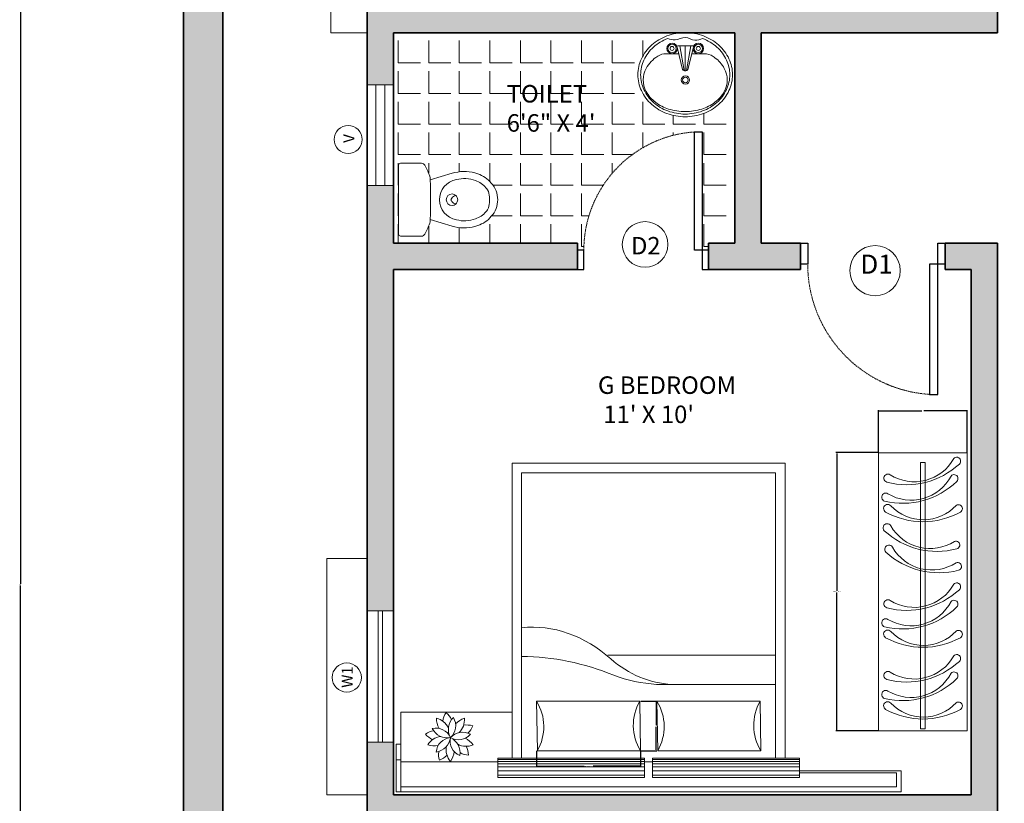
# Model space of a CAD drawing. Units: inches. Extents: x 2701 to 6846, y 811 to 2447.
# Tile 7 of 20: x 2701 to 2926, y 1130 to 1309. Entities that reach past the tile are written whole.
import ezdxf

# ---------------------------------------------------------------- set-up
doc = ezdxf.new("R2010")
doc.units = ezdxf.units.IN
doc.linetypes.add('HIDDEN4', pattern=[0.09375, 0.0625, -0.03125])
for name, color, linetype, lineweight in [('A-ANNO-DIMS', 2, 'Continuous', 18), ('A-ANNO-IDEN', 7, 'Continuous', 13), ('A-AREA-IDEN', 7, 'Continuous', 18), ('A-DOOR', 4, 'Continuous', 25), ('A-DOOR-SWNG', 4, 'HIDDEN4', 13), ('A-FLOR-FIXT', 7, 'Continuous', 18), ('A-FLOR-PATT', 252, 'Continuous', 13), ('A-FURN', 8, 'Continuous', 13), ('A-GLAZ', 4, 'Continuous', 18), ('A-WALL', 7, 'Continuous', 35), ('C-PROP', 7, 'Continuous', 35)]:
    doc.layers.add(name, color=color, linetype=linetype, lineweight=lineweight)
doc.layers.add('A-WALL-PATT', color=18, linetype='Continuous', lineweight=13, true_color=0x000000)
doc.layers.add('C-PROP-PATT', color=18, linetype='Continuous', lineweight=13, true_color=0x000000)
doc.styles.get("Standard").update_dxf_attribs({"font": 'arial.ttf'})
doc.dimstyles.get("Standard").update_dxf_attribs({"dimtxt": 0.18, "dimasz": 0.18, "dimexe": 0.18, "dimexo": 0.0625, "dimgap": 0.09, "dimtad": 0, "dimtih": 1, "dimtoh": 1, "dimdec": 4, "dimzin": 0, "dimdsep": 46, "dimtxsty": 'Standard', "dimcen": 0.09, "dimadec": 0, "dimazin": 0, "dimtfac": 1, "dimtdec": 4, "dimtofl": 0, "dimtmove": 0, "dimatfit": 3, "dimfxl": 1, "dimtolj": 1, "dimtzin": 0, "dimarcsym": 0})

# ---------------------------------------------------------------- blocks, each defined once
blk = doc.blocks.new('V')
for p, q in [((3304.15, 1279.33), (3281.15, 1279.33)), ((3304.15, 1277.33), (3281.15, 1277.33)), ((3304.15, 1275.33), (3281.15, 1275.33)), ((3281.15, 1273.33), (3304.15, 1273.33))]:
    blk.add_line(p, q)
blk.add_circle((3293.67, 1283.69), 3.19)
at = {"insert": (3292.45, 1284.76), "char_height": 2.5, "attachment_point": 1}
blk.add_mtext_dynamic_manual_height_columns('V', width=0.0153, gutter_width=12.5, heights=[0], dxfattribs=at)
blk = doc.blocks.new('V1')
for p, q in [((3281.15, 1279.33), (3281.15, 1273.33)), ((3304.15, 1273.33), (3304.15, 1279.33))]:
    blk.add_line(p, q)
blk.add_blockref('V', (0, 0))
blk = doc.blocks.new('A$C20D7642B')
for p, q in [((0, 1879.7), (0, 0)), ((600, 1879.7), (0, 1879.7)), ((600, 1879.7), (600, 0)), ((285.2, 14), (285.2, 1812.3)), ((285.2, 1812.3), (316, 1812.3)), ((316, 1812.3), (316, 14)), ((340, 0), (0, 0)), ((316, 14), (285.2, 14)), ((340, 0), (600, 0))]:
    blk.add_line(p, q)
for centre, radius, start, end in [((189.7, 2189.4), 526.2, 255.30638, 312.74923), ((242.6, 1988.3), 305.1, 237.78554, 330.91711), ((529.2, 1822.6), 26.4, 312.06888, 138.87685), ((64.5, 1707), 27.8, 56.33784, 252.73759), ((511.2, 1705.1), 26.4, 313.4541, 140.26207), ((163, 2063.5), 526.2, 256.69161, 314.13445), ((220.7, 1863.8), 305.1, 239.17077, 332.30233), ((49.5, 1578.3), 27.8, 57.72306, 254.12281), ((62.8, 1501.9), 27.8, 42.31003, 238.70978), ((301.2, 1939.5), 526.2, 241.27858, 298.72142), ((303.8, 1731.6), 305.1, 223.75774, 316.8893), ((541.6, 1501.4), 26.4, 298.04107, 124.84904), ((59.1, 1372.1), 27.8, 28.28014, 224.67989), ((396.5, 1738.9), 526.2, 227.24868, 284.69153), ((348.6, 1536.6), 305.1, 209.72784, 302.85941), ((523.6, 1255.6), 26.4, 284.01118, 110.81915), ((70.6, 1227.4), 27.8, 28.28014, 224.67989), ((408, 1594.2), 526.2, 227.24868, 284.69153), ((360, 1391.9), 305.1, 209.72784, 302.85941), ((535, 1110.9), 26.4, 284.01118, 110.81915), ((529.2, 973.6), 26.4, 312.06888, 138.87685), ((189.7, 1340.3), 526.2, 255.30638, 312.74923), ((242.6, 1139.3), 305.1, 237.78554, 330.91711), ((64.5, 857.9), 27.8, 56.33784, 252.73759), ((220.7, 1014.8), 305.1, 239.17077, 332.30233), ((511.2, 856), 26.4, 313.4541, 140.26207), ((163, 1214.5), 526.2, 256.69161, 314.13445), ((49.5, 729.2), 27.8, 57.72306, 254.12281), ((62.8, 652.8), 27.8, 42.31003, 238.70978), ((303.8, 882.6), 305.1, 223.75774, 316.8893), ((541.6, 652.4), 26.4, 298.04107, 124.84904), ((301.2, 1090.5), 526.2, 241.27858, 298.72142), ((189.7, 856), 526.2, 255.30638, 312.74923), ((242.6, 655), 305.1, 237.78554, 330.91711), ((529.2, 489.2), 26.4, 312.06888, 138.87685), ((64.5, 373.6), 27.8, 56.33784, 252.73759), ((163, 730.2), 526.2, 256.69161, 314.13445), ((220.7, 530.5), 305.1, 239.17077, 332.30233), ((511.2, 371.7), 26.4, 313.4541, 140.26207), ((49.5, 244.9), 27.8, 57.72306, 254.12281), ((62.8, 168.5), 27.8, 42.31003, 238.70978), ((301.2, 606.1), 526.2, 241.27858, 298.72142), ((303.8, 398.3), 305.1, 223.75774, 316.8893), ((541.6, 168), 26.4, 298.04107, 124.84904)]:
    blk.add_arc(centre, radius, start, end)
blk = doc.blocks.new('A$C62EA08CE')
at = {"linetype": 'ByBlock'}
for p, q in [((0.2191, 0.3943), (0.3067, 0.3943)), ((0.2328, 0.3943), (0.2566, 0.2566)), ((0.2629, 0.3943), (0.2629, 0.2555)), ((0.2933, 0.3943), (0.2696, 0.2568)), ((0.1569, 0.3505), (0.2264, 0.3505)), ((0.2191, 0.3797), (0.2483, 0.2629)), ((0.2775, 0.2629), (0.3067, 0.3797)), ((0.2994, 0.3505), (0.3691, 0.3505))]:
    blk.add_line(p, q, dxfattribs=at)
for centre, radius in [((0.1899, 0.3797), 0.0292), ((0.1899, 0.3797), 0.0232), ((0.1899, 0.3797), 0.0112), ((0.3359, 0.3797), 0.0292), ((0.3359, 0.3797), 0.0232), ((0.3359, 0.3797), 0.0112), ((0.264, 0.2045), 0.0234), ((0.264, 0.2045), 0.0154)]:
    blk.add_circle(centre, radius, dxfattribs=at)
for centre, radius, start, end in [((0.2518, 0.2022), 0.2632, 110.2132, 131.6335), ((0.2629, 0.1722), 0.2952, 90, 110.2132), ((0.2629, 0.1722), 0.2952, 69.7868, 90), ((0.2739, 0.2022), 0.2632, 48.3665, 69.7868), ((0.2348, 0.2214), 0.2375, 131.6335, 155.0149), ((0.2348, 0.2214), 0.2225, 131.6335, 155.0149), ((0.2518, 0.2022), 0.2482, 110.2132, 131.6335), ((0.2739, 0.2022), 0.2482, 48.3665, 69.7868), ((0.291, 0.2214), 0.2225, 24.9851, 48.3665), ((0.291, 0.2214), 0.2375, 24.9851, 48.3665), ((0.2107, 0.1777), 0.1883, 122.2598, 151.0888), ((0.1569, 0.2629), 0.0876, 90, 122.2598), ((0.3691, 0.2629), 0.0876, 56.0955, 90), ((0.2835, 0.1356), 0.241, 53.1301, 56.0955), ((0.2084, 0.2337), 0.2084, 155.0149, 180), ((0.2084, 0.2337), 0.1934, 155.0149, 180), ((0.3151, 0.1777), 0.1883, 28.9112, 53.1301), ((0.3174, 0.2337), 0.1934, 360, 24.9851), ((0.3174, 0.2337), 0.2084, 360, 24.9851), ((0.2084, 0.2337), 0.2084, 180, 204.9851), ((0.2084, 0.2337), 0.1934, 180, 204.9851), ((0.1622, 0.2045), 0.133, 151.0888, 180), ((0.2629, 0.2737), 0.0182, 216.4225, 323.5775), ((0.3636, 0.2045), 0.133, 0, 28.9112), ((0.3174, 0.2337), 0.1934, 335.0149, 0), ((0.3174, 0.2337), 0.2084, 335.0149, 0), ((0.1622, 0.2045), 0.133, 180, 208.9112), ((0.3636, 0.2045), 0.133, 331.0888, 0), ((0.2348, 0.246), 0.2375, 204.9851, 228.3665), ((0.2348, 0.246), 0.2225, 204.9851, 228.3665), ((0.2107, 0.2312), 0.1883, 208.9112, 233.1301), ((0.3151, 0.2312), 0.1883, 306.8699, 331.0888), ((0.291, 0.246), 0.2225, 311.6335, 335.0149), ((0.291, 0.246), 0.2375, 311.6335, 335.0149), ((0.2518, 0.2651), 0.2632, 228.3665, 249.7868), ((0.2518, 0.2651), 0.2482, 228.3665, 249.7868), ((0.2423, 0.2733), 0.241, 233.1301, 252.7421), ((0.2835, 0.2733), 0.241, 287.2579, 306.8699), ((0.2739, 0.2651), 0.2482, 290.2132, 311.6335), ((0.2739, 0.2651), 0.2632, 290.2132, 311.6335), ((0.2629, 0.2952), 0.2952, 249.7868, 270), ((0.2629, 0.2952), 0.2802, 249.7868, 270), ((0.2629, 0.3398), 0.3106, 252.7421, 270), ((0.2629, 0.3398), 0.3106, 270, 287.2579), ((0.2629, 0.2952), 0.2802, 270, 290.2132), ((0.2629, 0.2952), 0.2952, 270, 290.2132)]:
    blk.add_arc(centre, radius, start, end, dxfattribs=at)
blk.add_open_spline([(0.1661, 0.4351), (0.1795, 0.4306), (0.2124, 0.4195), (0.2631, 0.4543), (0.3132, 0.4162), (0.3455, 0.4293), (0.3597, 0.4351)], degree=3, knots=[0, 0, 0, 0, 0.0411087, 0.1003374, 0.1559132, 0.1995858, 0.1995858, 0.1995858, 0.1995858], dxfattribs=at)
blk = doc.blocks.new('A$C150B42AD')
at = {"ltscale": 20}
for p, q in [((0.243, 0.6605), (0.0125, 0.6605)), ((0.243, 0.6605), (0.4735, 0.6605)), ((0, 0.648), (0, 0.508)), ((0.486, 0.648), (0.486, 0.508)), ((0.11, 0.4499), (0.067, 0.3038)), ((0.1071, 0.45), (0.1511, 0.4485)), ((0.1511, 0.4485), (0.243, 0.4485)), ((0.3349, 0.4485), (0.243, 0.4485)), ((0.3789, 0.45), (0.3349, 0.4485)), ((0.376, 0.4499), (0.419, 0.3038)), ((0.2245, 0.0549), (0.243, 0.0549)), ((0.2615, 0.0549), (0.243, 0.0549))]:
    blk.add_line(p, q, dxfattribs=at)
for centre, radius, start, end in [((0.0125, 0.648), 0.0125, 90, 180), ((0.4735, 0.648), 0.0125, 0, 90), ((0.024, 0.508), 0.024, 180, 244), ((0.2288, 0.8612), 0.4323, 240.11805, 247.88195), ((0.1119, 0.5519), 0.102, 243.30484, 267.30484), ((0.3741, 0.5519), 0.102, 272.69516, 296.69516), ((0.2572, 0.8612), 0.4323, 292.11805, 299.88195), ((0.462, 0.508), 0.024, 296, 0), ((0.243, 0.252), 0.136, 90, 170.10936), ((0.243, 0.3047), 0.0384, 90, 270), ((0.243, 0.252), 0.136, 9.89064, 90), ((0.243, 0.3047), 0.0384, 270, 90), ((0.3111, 0.2222), 0.2565, 165.7118, 200.33768), ((0.243, 0.252), 0.1835, 163.59952, 169.46851), ((0.3111, 0.2222), 0.209, 165.27447, 200.60776), ((0.2251, 0.2822), 0.00957, 149.18444, 231.80771), ((0.2645, 0.2649), 0.0525, 119.17381, 155.01561), ((0.2439, 0.2978), 0.0139, 93.65397, 111.19045), ((0.2421, 0.2978), 0.0139, 68.80955, 86.34603), ((0.2215, 0.2649), 0.0525, 24.98439, 60.82619), ((0.2609, 0.2822), 0.00957, 308.19229, 30.81556), ((0.1749, 0.2222), 0.209, 339.39224, 14.72553), ((0.1749, 0.2222), 0.2565, 339.66232, 14.2882), ((0.243, 0.252), 0.1835, 10.53149, 16.40048), ((0.258, 0.194), 0.197, 198.0034, 230.27404), ((0.258, 0.194), 0.1495, 197.63909, 230.62819), ((0.228, 0.194), 0.1495, 309.37181, 342.36091), ((0.228, 0.194), 0.197, 309.72596, 341.9966), ((0.243, 0.166), 0.1185, 227.64547, 235.84675), ((0.2245, 0.1499), 0.095, 239.63238, 270), ((0.2615, 0.1499), 0.095, 270, 300.36762), ((0.243, 0.166), 0.1185, 304.15325, 312.35453), ((0.243, 0.166), 0.166, 228.0788, 270), ((0.243, 0.166), 0.166, 270, 311.9212)]:
    blk.add_arc(centre, radius, start, end, dxfattribs=at)
blk = doc.blocks.new('DOOR-D1-33IN-PANEL-FRAME')
blk.add_lwpolyline([(0, 33), (0, 31.37), (4.8, 31.37), (4.8, 33), (0, 33)], close=True)
for points in [[(4.32, 33), (0.48, 33)], [(4.8, 0), (4.8, 3.55), (34.54, 3.55), (34.54, 1.63), (0, 1.63), (0, 0)], [(0, 0), (4.8, 0)], [(4.32, 0), (0.48, 0)]]:
    blk.add_lwpolyline(points)
blk = doc.blocks.new('DOOR-D2-30IN-PANEL-FRAME')
blk.add_lwpolyline([(0, 30), (0, 28.52), (4.36, 28.52), (4.36, 30), (0, 30)], close=True)
for points in [[(3.93, 30), (0.44, 30)], [(4.36, 0), (4.36, 3.22), (31.4, 3.22), (31.4, 1.48), (0, 1.48), (0, 0)], [(0, 0), (4.36, 0)], [(3.93, 0), (0.44, 0)]]:
    blk.add_lwpolyline(points)
blk = doc.blocks.new('BED-PILLOW')
for p, q in [((23.58, 11.3), (0, 11.3)), ((0, 11.3), (0.17, 0)), ((23.75, 0), (23.58, 11.3)), ((0.17, 0), (23.75, 0))]:
    blk.add_line(p, q)
for centre, start, end in [((-9.32, 5.51), 329.8722, 31.8713), ((33.07, 5.79), 149.8722, 211.8713)]:
    blk.add_arc(centre, 10.97, start, end)
blk = doc.blocks.new('*D43')
at = {"layer": 'A-ANNO-DIMS', "color": 0, "lineweight": -2, "transparency": 16777216}
for p, q in [((2896.7, 1210.2), (2887.05, 1210.2)), ((2887.23, 1210.02), (2887.23, 1178.62)), ((2887.23, 1146.85), (2887.23, 1178.25)), ((2896.7, 1146.67), (2887.05, 1146.67))]:
    blk.add_line(p, q, dxfattribs=at)
at = {"layer": 'A-ANNO-DIMS', "color": 0, "transparency": 16777216}
for points in [[(2887.2, 1210.02), (2887.26, 1210.02), (2887.23, 1210.2)], [(2887.2, 1146.85), (2887.26, 1146.85), (2887.23, 1146.67)]]:
    blk.add_solid(points, dxfattribs=at)
at = {"layer": 'Defpoints', "color": 0, "transparency": 16777216}
for p in [(2887.23, 1210.2), (2896.76, 1210.2), (2896.76, 1146.67)]:
    blk.add_point(p, dxfattribs=at)
at = {"layer": 'A-ANNO-DIMS', "color": 0, "transparency": 16777216, "insert": (2887.23, 1178.44), "char_height": 0.18, "attachment_point": 5}
blk.add_mtext('\\A1;WARDROBE 64', dxfattribs=at)
blk = doc.blocks.new('*D44')
at = {"layer": 'A-ANNO-DIMS', "color": 0, "lineweight": -2, "transparency": 16777216}
for p, q in [((2896.76, 1210.26), (2896.76, 1219.91)), ((2896.94, 1219.73), (2906.68, 1219.73)), ((2916.86, 1219.73), (2907.12, 1219.73)), ((2917.04, 1210.26), (2917.04, 1219.91))]:
    blk.add_line(p, q, dxfattribs=at)
at = {"layer": 'A-ANNO-DIMS', "color": 0, "transparency": 16777216}
for points in [[(2896.94, 1219.76), (2896.94, 1219.7), (2896.76, 1219.73)], [(2916.86, 1219.76), (2916.86, 1219.7), (2917.04, 1219.73)]]:
    blk.add_solid(points, dxfattribs=at)
at = {"layer": 'Defpoints', "color": 0, "transparency": 16777216}
for p in [(2917.04, 1219.73), (2896.76, 1210.2), (2917.04, 1210.2)]:
    blk.add_point(p, dxfattribs=at)
at = {"layer": 'A-ANNO-DIMS', "color": 0, "transparency": 16777216, "insert": (2906.9, 1219.73), "char_height": 0.18, "attachment_point": 5}
blk.add_mtext('\\A1;20', dxfattribs=at)
blk = doc.blocks.new('*D47')
at = {"layer": 'A-ANNO-DIMS', "color": 0, "lineweight": -2, "transparency": 16777216}
for p, q in [((2818.66, 1142.07), (2818.66, 1138.39)), ((2842.41, 1142.07), (2842.41, 1138.39)), ((2818.84, 1138.57), (2829.5, 1138.57)), ((2842.23, 1138.57), (2831.57, 1138.57))]:
    blk.add_line(p, q, dxfattribs=at)
at = {"layer": 'A-ANNO-DIMS', "color": 0, "transparency": 16777216}
for points in [[(2818.84, 1138.6), (2818.84, 1138.54), (2818.66, 1138.57)], [(2842.23, 1138.6), (2842.23, 1138.54), (2842.41, 1138.57)]]:
    blk.add_solid(points, dxfattribs=at)
at = {"layer": 'Defpoints', "color": 0, "transparency": 16777216}
for p in [(2818.66, 1142.13), (2842.41, 1142.13), (2842.41, 1138.57)]:
    blk.add_point(p, dxfattribs=at)
at = {"layer": 'A-ANNO-DIMS', "color": 0, "transparency": 16777216, "insert": (2830.53, 1138.57), "char_height": 0.18, "attachment_point": 5}
blk.add_mtext('\\A1;PILLOW 24 TYP.', dxfattribs=at)
blk = doc.blocks.new('*D48')
at = {"layer": 'A-ANNO-DIMS', "color": 0, "lineweight": -2, "transparency": 16777216}
for p, q in [((2842.47, 1153.44), (2846.15, 1153.44)), ((2845.97, 1153.26), (2845.97, 1147.97)), ((2845.97, 1142.31), (2845.97, 1147.61)), ((2842.47, 1142.13), (2846.15, 1142.13))]:
    blk.add_line(p, q, dxfattribs=at)
at = {"layer": 'A-ANNO-DIMS', "color": 0, "transparency": 16777216}
for points in [[(2845.94, 1153.26), (2846, 1153.26), (2845.97, 1153.44)], [(2845.94, 1142.31), (2846, 1142.31), (2845.97, 1142.13)]]:
    blk.add_solid(points, dxfattribs=at)
at = {"layer": 'Defpoints', "color": 0, "transparency": 16777216}
for p in [(2842.41, 1153.44), (2845.97, 1153.44), (2842.41, 1142.13)]:
    blk.add_point(p, dxfattribs=at)
at = {"layer": 'A-ANNO-DIMS', "color": 0, "transparency": 16777216, "insert": (2845.97, 1147.79), "char_height": 0.18, "attachment_point": 5}
blk.add_mtext('\\A1;11 TYP.', dxfattribs=at)
blk = doc.blocks.new('*D66')
at = {"layer": 'A-ANNO-DIMS', "color": 0, "lineweight": -2, "transparency": 16777216}
for p, q in [((2737.91, 1504.05), (2700.59, 1504.05)), ((2700.77, 1503.87), (2700.77, 1180.23)), ((2700.77, 856.23), (2700.77, 1179.87)), ((2737.91, 856.05), (2700.59, 856.05))]:
    blk.add_line(p, q, dxfattribs=at)
at = {"layer": 'A-ANNO-DIMS', "color": 0, "transparency": 16777216}
for points in [[(2700.74, 1503.87), (2700.8, 1503.87), (2700.77, 1504.05)], [(2700.74, 856.23), (2700.8, 856.23), (2700.77, 856.05)]]:
    blk.add_solid(points, dxfattribs=at)
at = {"layer": 'Defpoints', "color": 0, "transparency": 16777216}
for p in [(2700.77, 1504.05), (2737.97, 1504.05), (2737.97, 856.05)]:
    blk.add_point(p, dxfattribs=at)
at = {"layer": 'A-ANNO-DIMS', "color": 0, "transparency": 16777216, "insert": (2700.77, 1180.05), "char_height": 0.18, "attachment_point": 5}
blk.add_mtext('\\A1;648', dxfattribs=at)

msp = doc.modelspace()

# ---------------------------------------------------------------- hatches: boundary and pattern name
at = {"layer": 'A-FLOR-PATT'}
h = msp.add_hatch(dxfattribs=at)
h.set_pattern_fill('ANGLE', color=256)
h.set_pattern_definition([(0, (0, 0), (0, 6.985), [5.08, -1.905]), (90, (0, 0), (-6.985, 4e-16), [5.08, -1.905])])
h.paths.add_polyline_path([(2841.81, 1296.51, -0.109453), (2842.61, 1300.13, -0.102375), (2844.98, 1303.3, -0.093743), (2848.43, 1305.37, -0.062463), (2851.37, 1306.05), (2785.97, 1306.05), (2785.97, 1258.05), (2827.97, 1258.05), (2827.97, 1256.41), (2829.45, 1256.41, -0.394827), (2854.75, 1283.45), (2856.49, 1283.45), (2856.49, 1256.41), (2857.97, 1256.41), (2857.97, 1258.05), (2863.97, 1258.05), (2863.97, 1306.05), (2853.87, 1306.05, -0.062463), (2856.81, 1305.37, -0.093743), (2860.26, 1303.3, -0.102375), (2862.62, 1300.13, -0.109453), (2863.42, 1296.51, -0.109453), (2862.62, 1292.89, -0.102375), (2860.26, 1289.72, -0.093738), (2856.81, 1287.65, -0.088425), (2852.62, 1286.91, -0.088425), (2848.43, 1287.65, -0.093738), (2844.98, 1289.72, -0.102375), (2842.61, 1292.89, -0.109453)])
h.paths.add_polyline_path([(2805.21, 1273.88, -0.141745), (2808.32, 1271.77, -0.184983), (2809.77, 1267.97, -0.184983), (2808.32, 1264.18, -0.141745), (2805.21, 1262.07, -0.152244), (2799.99, 1261.8, -0.025614), (2799.37, 1261.95), (2794.37, 1263.42), (2794.36, 1263.41, -0.111242), (2793.99, 1261.92, -0.033889), (2793.11, 1260.11, -0.286745), (2792.38, 1259.65), (2787.58, 1259.65, -0.414214), (2787.15, 1260.08), (2787.15, 1267.97), (2787.15, 1275.87, -0.414214), (2787.58, 1276.3), (2792.38, 1276.3, -0.286745), (2793.11, 1275.83, -0.033889), (2793.99, 1274.03, -0.105104), (2794.36, 1272.63), (2794.37, 1272.53), (2799.37, 1274, -0.025614), (2799.99, 1274.15, -0.152244)], flags=16)
h.paths.add_polyline_path([(2804.68, 1272.34, -0.144945), (2807.09, 1270.71, -0.0358), (2807.45, 1270.25, -0.133285), (2807.89, 1268.61), (2807.89, 1267.97), (2807.89, 1267.34, -0.133285), (2807.45, 1265.7, -0.0358), (2807.09, 1265.24, -0.144945), (2804.68, 1263.61, -0.155404), (2800.34, 1263.39, -0.364511), (2796.49, 1267.97, -0.364511), (2800.34, 1272.56, -0.155404)], flags=0)
h.paths.add_polyline_path([(2800.02, 1268.9, 0.169298), (2799.13, 1268.12, 0.076667), (2799.1, 1267.97, 0.076667), (2799.13, 1267.83, 0.169298), (2800.02, 1267.05, 0.305219), (2800.37, 1267.16, 0.169535), (2800.65, 1267.97, 0.169535), (2800.37, 1268.79, 0.305219)], flags=0)
h.paths.add_polyline_path([(2971.97, 1456.05), (2923.97, 1456.05), (2923.97, 1408.05), (2922.33, 1408.05), (2922.33, 1406.57, -0.394827), (2949.37, 1381.27), (2949.37, 1379.53), (2922.33, 1379.53), (2922.33, 1378.05), (2923.97, 1378.05), (2923.97, 1372.05), (2971.97, 1372.05)])
h.paths.add_polyline_path([(2939.82, 1436.53, -0.141745), (2937.71, 1433.42, -0.184983), (2933.91, 1431.97, -0.184983), (2930.12, 1433.42, -0.141745), (2928.01, 1436.53, -0.152244), (2927.74, 1441.75, -0.025614), (2927.89, 1442.37), (2929.36, 1447.38), (2929.35, 1447.38, -0.111242), (2927.86, 1447.75, -0.033889), (2926.05, 1448.63, -0.286745), (2925.59, 1449.37), (2925.59, 1454.16, -0.414214), (2926.02, 1454.59), (2933.91, 1454.59), (2941.81, 1454.59, -0.414207), (2942.24, 1454.16), (2942.24, 1449.37, -0.286745), (2941.78, 1448.63, -0.033889), (2939.97, 1447.75, -0.105104), (2938.57, 1447.38), (2938.47, 1447.38), (2939.94, 1442.37, -0.025614), (2940.09, 1441.75, -0.152244)], flags=16)
h.paths.add_polyline_path([(2938.28, 1437.06, -0.144945), (2936.65, 1434.65, -0.0358), (2936.19, 1434.29, -0.133285), (2934.55, 1433.85), (2933.91, 1433.85), (2933.28, 1433.85, -0.133285), (2931.64, 1434.29, -0.0358), (2931.18, 1434.65, -0.144945), (2929.55, 1437.06, -0.155404), (2929.33, 1441.4, -0.364511), (2933.91, 1445.26, -0.364511), (2938.5, 1441.4, -0.155404)], flags=0)
h.paths.add_polyline_path([(2969.16, 1392.04, -0.093743), (2971.22, 1388.6, -0.088421), (2971.97, 1384.4, -0.088421), (2971.22, 1380.21, -0.093743), (2969.16, 1376.76, -0.102375), (2965.99, 1374.4, -0.109453), (2962.37, 1373.6, -0.109453), (2958.75, 1374.4, -0.102375), (2955.58, 1376.76, -0.093738), (2953.51, 1380.21, -0.088425), (2952.76, 1384.4, -0.088425), (2953.51, 1388.6, -0.093738), (2955.58, 1392.04, -0.102375), (2958.75, 1394.41, -0.109453), (2962.37, 1395.21, -0.109453), (2965.99, 1394.41, -0.102375)], flags=0)
edge = h.paths.add_edge_path(flags=16)
edge.add_arc((2961.07, 1384.86), 10.2, 20.2132, 41.6336, ccw=False)
edge.add_spline(control_points=[(2970.65, 1388.38), (2970.46, 1387.83), (2970, 1386.48), (2971.44, 1384.4), (2969.87, 1382.34), (2970.41, 1381.01), (2970.65, 1380.43)], knot_values=[0, 0, 0, 0, 0.041109, 0.100337, 0.155913, 0.199586, 0.199586, 0.199586, 0.199586], degree=3, periodic=0)
edge.add_arc((2961.07, 1383.95), 10.2, 318.3664, 339.7868, ccw=False)
edge.add_arc((2961.86, 1383.25), 9.15, 294.9853, 318.3664, ccw=False)
edge.add_arc((2962.37, 1382.17), 7.95, 270, 294.9853, ccw=False)
edge.add_arc((2962.37, 1382.17), 7.95, 245.0147, 270, ccw=False)
edge.add_arc((2962.87, 1383.25), 9.15, 221.6336, 245.0147, ccw=False)
edge.add_arc((2963.66, 1383.95), 10.2, 200.213, 221.6336, ccw=False)
edge.add_arc((2964.89, 1384.4), 11.51, 180, 200.213, ccw=False)
edge.add_arc((2964.89, 1384.4), 11.51, 159.787, 180, ccw=False)
edge.add_arc((2963.66, 1384.86), 10.2, 138.3664, 159.787, ccw=False)
edge.add_arc((2962.87, 1385.56), 9.15, 114.9853, 138.3664, ccw=False)
edge.add_arc((2962.37, 1386.64), 7.95, 90, 114.9853, ccw=False)
edge.add_arc((2962.37, 1386.64), 7.95, 65.0147, 90, ccw=False)
edge.add_arc((2961.86, 1385.56), 9.15, 41.6336, 65.0147, ccw=False)
h.paths.add_polyline_path([(2963.81, 1393.33, -0.126458), (2966.61, 1390.68, -0.141697), (2967.17, 1388.76), (2967.17, 1387.41, -1), (2969.57, 1387.41, -0.414214), (2968.37, 1386.21), (2963.57, 1385, 0.146218), (2963.31, 1384.66), (2968.97, 1385.64), (2968.97, 1383.15), (2963.32, 1384.13, 0.140312), (2963.57, 1383.8), (2968.37, 1382.6, -0.414214), (2969.57, 1381.4, -1), (2967.17, 1381.4), (2967.17, 1380.04, -0.149025), (2966.56, 1378.03, -0.012759), (2966.26, 1377.62, -0.106303), (2963.81, 1375.48, -0.126822), (2961.17, 1374.8, -0.126822), (2958.52, 1375.48, -0.106303), (2956.07, 1377.62, -0.085722), (2954.54, 1380.62, -0.075351), (2953.96, 1384.4, -0.075351), (2954.54, 1388.19, -0.085722), (2956.07, 1391.19, -0.106303), (2958.52, 1393.33, -0.126822), (2961.17, 1394.01, -0.126822)], flags=0)
h.paths.add_polyline_path([(2934.84, 1441.73, 0.169298), (2934.06, 1442.61, 0.076667), (2933.91, 1442.64, 0.076667), (2933.77, 1442.61, 0.169298), (2932.99, 1441.73, 0.305219), (2933.1, 1441.38, 0.169535), (2933.91, 1441.09, 0.169535), (2934.73, 1441.38, 0.305219)], flags=0)
h.paths.add_polyline_path([(2969.32, 1387.41, -1), (2967.42, 1387.41, -1)], flags=0)
h.paths.add_polyline_path([(2968.83, 1387.41, -1), (2967.91, 1387.41, -1)], flags=0)
h.paths.add_polyline_path([(2962.13, 1384.36, -1), (2960.21, 1384.36, -1)], flags=0)
h.paths.add_polyline_path([(2961.8, 1384.36, -1), (2960.54, 1384.36, -1)], flags=0)
h.paths.add_polyline_path([(2969.32, 1381.4, -1), (2967.42, 1381.4, -1)], flags=0)
h.paths.add_polyline_path([(2968.83, 1381.4, -1), (2967.91, 1381.4, -1)], flags=0)
h.paths.add_polyline_path([(3085.97, 1306.05), (3001.97, 1306.05), (3001.97, 1300.05), (3000.33, 1300.05), (3000.33, 1298.57), (3027.37, 1298.57), (3027.37, 1296.83, -0.394827), (3000.33, 1271.53), (3000.33, 1270.05), (3001.97, 1270.05), (3001.97, 1258.05), (3085.97, 1258.05)])
h.paths.add_polyline_path([(3033.33, 1274.44, -0.102375), (3035.7, 1271.27, -0.109453), (3036.5, 1267.65, -0.109453), (3035.7, 1264.04, -0.102375), (3033.33, 1260.86, -0.093743), (3029.88, 1258.8, -0.088421), (3025.69, 1258.05, -0.088421), (3021.5, 1258.8, -0.093743), (3018.05, 1260.86, -0.102375), (3015.69, 1264.04, -0.109453), (3014.89, 1267.65, -0.109453), (3015.69, 1271.27, -0.102375), (3018.05, 1274.44, -0.093738), (3021.5, 1276.51, -0.088425), (3025.69, 1277.26, -0.088425), (3029.88, 1276.51, -0.093738)], flags=0)
edge = h.paths.add_edge_path(flags=16)
edge.add_arc((3026.85, 1267.15), 9.15, 24.9853, 48.3664, ccw=False)
edge.add_arc((3027.93, 1267.65), 7.95, 0, 24.9853, ccw=False)
edge.add_arc((3027.93, 1267.65), 7.95, -24.9853, 0, ccw=False)
edge.add_arc((3026.85, 1268.16), 9.15, 311.6336, 335.0147, ccw=False)
edge.add_arc((3026.15, 1268.95), 10.2, 290.2132, 311.6336, ccw=False)
edge.add_spline(control_points=[(3029.67, 1259.38), (3029.09, 1259.61), (3027.76, 1260.15), (3025.7, 1258.59), (3023.62, 1260.02), (3022.27, 1259.56), (3021.71, 1259.38)], knot_values=[0, 0, 0, 0, 0.043673, 0.099248, 0.158477, 0.199586, 0.199586, 0.199586, 0.199586], degree=3, periodic=0)
edge.add_arc((3025.24, 1268.95), 10.2, 228.3664, 249.7868, ccw=False)
edge.add_arc((3024.54, 1268.16), 9.15, 204.9853, 228.3664, ccw=False)
edge.add_arc((3023.45, 1267.65), 7.95, 180, 204.9853, ccw=False)
edge.add_arc((3023.45, 1267.65), 7.95, 155.0147, 180, ccw=False)
edge.add_arc((3024.54, 1267.15), 9.15, 131.6336, 155.0147, ccw=False)
edge.add_arc((3025.24, 1266.36), 10.2, 110.213, 131.6336, ccw=False)
edge.add_arc((3025.69, 1265.13), 11.51, 90, 110.213, ccw=False)
edge.add_arc((3025.69, 1265.13), 11.51, 69.787, 90, ccw=False)
edge.add_arc((3026.15, 1266.36), 10.2, 48.3664, 69.787, ccw=False)
h.paths.add_polyline_path([(3032.48, 1273.95, -0.106303), (3034.62, 1271.5, -0.126822), (3035.3, 1268.85, -0.126822), (3034.62, 1266.21, -0.106303), (3032.48, 1263.76, -0.012759), (3032.07, 1263.46, -0.149025), (3030.06, 1262.85), (3028.69, 1262.85, -0.414214), (3029.89, 1261.65, -1), (3027.49, 1261.65), (3026.29, 1266.45, 0.140312), (3025.97, 1266.7), (3026.94, 1261.05), (3024.46, 1261.05), (3025.43, 1266.71, 0.146218), (3025.09, 1266.45), (3023.89, 1261.65, -1), (3021.49, 1261.65, -0.414214), (3022.69, 1262.85), (3021.34, 1262.85, -0.141697), (3019.41, 1263.41, -0.126458), (3016.77, 1266.21, -0.126822), (3016.09, 1268.85, -0.126822), (3016.77, 1271.5, -0.106303), (3018.91, 1273.95, -0.085722), (3021.91, 1275.48, -0.075351), (3025.69, 1276.06, -0.075351), (3029.47, 1275.48, -0.085722)], flags=0)
h.paths.add_polyline_path([(3072.36, 1280, -0.184983), (3076.16, 1281.46, -0.184983), (3079.96, 1280, -0.141745), (3082.07, 1276.9, -0.152244), (3082.34, 1271.68, -0.025614), (3082.19, 1271.05), (3080.72, 1266.05), (3080.82, 1266.04, -0.105104), (3082.22, 1265.68, -0.033889), (3084.02, 1264.8, -0.286745), (3084.49, 1264.06), (3084.49, 1259.26, -0.41422), (3084.06, 1258.84), (3076.16, 1258.84), (3068.27, 1258.84, -0.414214), (3067.84, 1259.26), (3067.84, 1264.06, -0.286745), (3068.3, 1264.8, -0.033889), (3070.1, 1265.68, -0.105104), (3071.51, 1266.04), (3071.61, 1266.05), (3070.13, 1271.05, -0.025614), (3069.98, 1271.68, -0.152244), (3070.26, 1276.9, -0.141745)], flags=16)
h.paths.add_polyline_path([(3073.43, 1278.77, -0.0358), (3073.88, 1279.13, -0.133285), (3075.53, 1279.58), (3076.16, 1279.58), (3076.8, 1279.58, -0.133285), (3078.44, 1279.13, -0.0358), (3078.9, 1278.77, -0.144945), (3080.53, 1276.36, -0.155404), (3080.75, 1272.03, -0.364511), (3076.16, 1268.17, -0.364511), (3071.57, 1272.03, -0.155404), (3071.8, 1276.36, -0.144945)], flags=0)
h.paths.add_polyline_path([(3026.7, 1268.85, -1), (3024.78, 1268.85, -1)], flags=0)
h.paths.add_polyline_path([(3026.37, 1268.85, -1), (3025.11, 1268.85, -1)], flags=0)
h.paths.add_polyline_path([(3075.27, 1271.62, 0.157677), (3076.02, 1270.81, 0.076667), (3076.16, 1270.78, 0.076667), (3076.3, 1270.81, 0.157677), (3077.06, 1271.62, 0.374626), (3076.98, 1272.05, 0.169535), (3076.16, 1272.33, 0.169535), (3075.35, 1272.05, 0.374626)], flags=0)
h.paths.add_polyline_path([(3029.65, 1261.65, -1), (3027.74, 1261.65, -1)], flags=0)
h.paths.add_polyline_path([(3029.15, 1261.65, -1), (3028.23, 1261.65, -1)], flags=0)
h.paths.add_polyline_path([(3023.65, 1261.65, -1), (3021.74, 1261.65, -1)], flags=0)
h.paths.add_polyline_path([(3023.15, 1261.65, -1), (3022.23, 1261.65, -1)], flags=0)
h.paths.add_polyline_path([(2810.57, 1281.22), (2833.31, 1281.22), (2833.31, 1296.43), (2810.57, 1296.43)], flags=24)
h.paths.add_polyline_path([(2937.55, 1410.24), (2960.21, 1410.24), (2960.21, 1425.45), (2937.55, 1425.45)], flags=24)
h.paths.add_polyline_path([(3043.23, 1273.1), (3065.89, 1273.1), (3065.89, 1288.31), (3043.23, 1288.31)], flags=24)
at = {"layer": 'A-WALL-PATT'}
h = msp.add_hatch(color=256, dxfattribs=at)
h.dxf.hatch_style = 1
h.paths.add_polyline_path([(3085.97, 1456.05), (3085.97, 1348.05), (3091.97, 1348.05), (3091.97, 1360.05), (3091.97, 1462.05), (2960.09, 1462.05), (2960.09, 1456.05), (2971.97, 1456.05), (2971.97, 1372.05), (2923.97, 1372.05), (2923.97, 1378.05), (2917.97, 1378.05), (2917.97, 1351.05), (2923.97, 1351.05), (2923.97, 1366.05), (2971.97, 1366.05), (2971.97, 1351.05), (2976.77, 1351.05), (2977.97, 1351.05), (2977.97, 1456.05)])
h.paths.add_polyline_path([(2779.97, 1462.05), (2779.97, 1342.05), (2785.97, 1342.05), (2785.97, 1456.05), (2917.97, 1456.05), (2917.97, 1408.05), (2922.33, 1408.05), (2923.97, 1408.05), (2923.97, 1456.05), (2937.09, 1456.05), (2937.09, 1462.05)])
h.paths.add_polyline_path([(2779.97, 1306.05), (2779.97, 1294.24), (2785.97, 1294.24), (2785.97, 1306.05), (2851.37, 1306.05, -0.025815), (2852.62, 1306.11, -0.025815), (2853.87, 1306.05), (2863.97, 1306.05), (2863.97, 1258.05), (2857.97, 1258.05), (2857.97, 1252.05), (2878.97, 1252.05), (2878.97, 1258.05), (2869.97, 1258.05), (2869.97, 1306.05), (2923.97, 1306.05), (2923.97, 1318.05), (2919.17, 1318.05), (2917.97, 1318.05), (2917.97, 1312.05), (2785.97, 1312.05), (2785.97, 1318.05), (2779.97, 1318.05)])
h.paths.add_polyline_path([(2785.97, 1252.05), (2827.97, 1252.05), (2827.97, 1256.41), (2827.97, 1258.05), (2785.97, 1258.05), (2785.97, 1271.24), (2779.97, 1271.24), (2779.97, 1174.05), (2785.97, 1174.05)])
h.paths.add_polyline_path([(2779.97, 1030.05), (2869.97, 1030.05), (2869.97, 1036.05), (2785.97, 1036.05), (2785.97, 1126.05), (2917.97, 1126.05), (2917.97, 1120.05), (2923.97, 1120.05), (2923.97, 1258.05), (2911.97, 1258.05), (2911.97, 1253.25), (2911.97, 1252.05), (2917.97, 1252.05), (2917.97, 1132.05), (2785.97, 1132.05), (2785.97, 1144.05), (2779.97, 1144.05)])
h.paths.add_polyline_path([(2935.97, 1030.05), (2935.97, 1033.05), (2935.97, 1036.05), (2923.97, 1036.05), (2923.97, 1087.05), (2919.17, 1087.05), (2917.97, 1087.05), (2917.97, 1036.05), (2893.97, 1036.05), (2893.97, 1030.05)])
h.paths.add_polyline_path([(2971.97, 1036.05), (2971.97, 1030.05), (3091.97, 1030.05), (3091.97, 1060.05), (3085.97, 1060.05), (3085.97, 1036.05)])
h.paths.add_polyline_path([(3085.97, 1084.05), (3091.97, 1084.05), (3091.97, 1096.05), (3091.97, 1268.89), (3085.97, 1268.89), (3085.97, 1258.05), (3001.97, 1258.05), (3001.97, 1270.05), (2995.97, 1270.05), (2995.97, 1252.05), (3085.97, 1252.05)])
h.paths.add_polyline_path([(3085.97, 1306.05), (3085.97, 1291.89), (3091.97, 1291.89), (3091.97, 1318.05), (3085.97, 1318.05), (3085.97, 1312.05), (2977.97, 1312.05), (2977.97, 1318.05), (2971.97, 1318.05), (2971.97, 1306.05), (2995.97, 1306.05), (2995.97, 1300.05), (3000.33, 1300.05), (3001.97, 1300.05), (3001.97, 1306.05)])
at = {"layer": 'C-PROP-PATT'}
h = msp.add_hatch(color=256, dxfattribs=at)
h.dxf.hatch_style = 1
h.paths.add_polyline_path([(3145.97, 1504.05), (2737.97, 1504.05), (2737.97, 967.05), (2746.97, 967.05), (2746.97, 1495.05), (3136.97, 1495.05), (3136.97, 865.05), (3130.97, 865.05), (3130.97, 856.05), (3145.97, 856.05)])
h.paths.add_polyline_path([(3070.97, 865.05), (2746.97, 865.05), (2746.97, 871.05), (2737.97, 871.05), (2737.97, 856.05), (3070.97, 856.05)], flags=17)

# ---------------------------------------------------------------- linework, layer by layer
at = {"layer": 'A-ANNO-IDEN'}
for centre, radius in [((2843.44, 1257.76), 5.22), ((2895.99, 1251.77), 5.74), ((2775.29, 1158.84), 3.33)]:
    msp.add_circle(centre, radius, dxfattribs=at)
at = {"layer": 'A-DOOR-SWNG'}
for centre, radius, start, end in [((2856.55, 1256.41), 27.1, 93.8183, 180), ((2910.41, 1253.25), 29.81, 180, 266.1817)]:
    msp.add_arc(centre, radius, start, end, dxfattribs=at)
at = {"layer": 'A-FURN'}
for p, q in [((2875.45, 1207.78), (2813.06, 1207.78)), ((2813.06, 1150.91), (2813.06, 1207.78)), ((2875.45, 1150.91), (2875.45, 1207.78)), ((2873.28, 1205.61), (2815.24, 1205.61)), ((2815.24, 1140.39), (2815.24, 1205.61)), ((2873.28, 1140.39), (2873.28, 1205.61)), ((2834.91, 1163.92), (2873.28, 1163.92)), ((2846.07, 1157.28), (2873.28, 1157.28)), ((2787.67, 1150.91), (2787.67, 1143.65)), ((2787.67, 1150.91), (2813.06, 1150.91)), ((2813.06, 1150.91), (2813.06, 1140.39)), ((2875.45, 1150.91), (2875.45, 1140.39)), ((2786.58, 1132.77), (2786.58, 1143.65)), ((2786.58, 1143.65), (2787.67, 1143.65)), ((2787.67, 1143.65), (2787.67, 1132.77)), ((2787.67, 1140.03), (2786.58, 1140.03)), ((2787.67, 1139.59), (2809.8, 1139.59)), ((2809.8, 1136.04), (2809.8, 1140.39)), ((2843.35, 1140.39), (2809.8, 1140.39)), ((2843.35, 1140.09), (2809.8, 1140.09)), ((2843.35, 1139.69), (2809.8, 1139.69)), ((2843.35, 1139.13), (2809.8, 1139.13)), ((2843.35, 1138.41), (2809.8, 1138.41)), ((2843.35, 1136.04), (2843.35, 1140.39)), ((2845.17, 1139.59), (2843.35, 1139.59)), ((2878.72, 1140.39), (2845.17, 1140.39)), ((2845.17, 1136.04), (2845.17, 1140.39)), ((2878.72, 1140.09), (2845.17, 1140.09)), ((2878.72, 1139.69), (2845.17, 1139.69)), ((2878.72, 1139.13), (2845.17, 1139.13)), ((2878.72, 1138.41), (2845.17, 1138.41)), ((2878.72, 1136.04), (2878.72, 1140.39)), ((2843.35, 1137.54), (2809.8, 1137.54)), ((2843.35, 1136.58), (2809.8, 1136.58)), ((2843.35, 1136.04), (2809.8, 1136.04)), ((2878.72, 1137.54), (2845.17, 1137.54)), ((2878.72, 1136.58), (2845.17, 1136.58)), ((2878.72, 1136.04), (2845.17, 1136.04)), ((2901.93, 1137.54), (2878.72, 1137.54)), ((2900.85, 1137.04), (2878.72, 1137.04)), ((2900.85, 1133.86), (2900.85, 1137.04)), ((2901.93, 1132.77), (2901.93, 1137.54)), ((2787.67, 1133.86), (2809.8, 1133.86)), ((2843.35, 1133.86), (2809.8, 1133.86)), ((2845.17, 1133.86), (2843.35, 1133.86)), ((2878.72, 1133.86), (2845.17, 1133.86)), ((2900.85, 1133.86), (2878.72, 1133.86)), ((2809.8, 1132.77), (2786.58, 1132.77)), ((2843.35, 1132.77), (2809.8, 1132.77)), ((2901.93, 1132.77), (2843.35, 1132.77))]:
    msp.add_line(p, q, dxfattribs=at)
for centre, radius, start, end in [((2800.31, 1149.47), 4.53, 179.1301, 209.4932), ((2794.81, 1145.47), 4.18, 27.1324, 76.6013), ((2802.76, 1147.85), 5.64, 148.2105, 169.3514), ((2795.97, 1147.93), 3.51, 21.5086, 55.2476), ((2802.36, 1146.98), 3.85, 134.7761, 208.5159), ((2796.64, 1147.82), 3.55, 311.0447, 32.2473), ((2803.51, 1145.21), 4.53, 107.1301, 137.4932), ((2798, 1149.21), 4.18, 315.1324, 4.6013), ((2795.7, 1143.75), 3.55, 23.0447, 104.2473), ((2802.72, 1142.37), 5.64, 76.2105, 97.3514), ((2800.7, 1148.86), 3.51, 309.5086, 343.2476), ((2795.39, 1143.14), 3.51, 93.5086, 127.2476), ((2797.57, 1149.58), 5.64, 220.2105, 241.3514), ((2797.37, 1141.28), 4.18, 99.1324, 148.6013), ((2798.27, 1148.93), 3.85, 206.7761, 280.5159), ((2795.15, 1145.64), 3.85, 278.7761, 352.5159), ((2799.29, 1141.6), 3.55, 95.0447, 176.2473), ((2802.44, 1144.34), 3.55, 167.0447, 248.2473), ((2801.77, 1142.49), 3.85, 62.7761, 136.5159), ((2800.8, 1148.19), 3.55, 239.0447, 320.2473), ((2797.32, 1141.66), 3.85, 350.7761, 64.5159), ((2795.27, 1147.75), 4.53, 251.1301, 281.4931), ((2802.15, 1142.42), 4.18, 171.1324, 220.6013), ((2802.54, 1147.32), 4.18, 243.1324, 292.6013), ((2800.44, 1140.85), 4.53, 35.1301, 65.4931), ((2797.5, 1140.72), 5.64, 4.2105, 25.3514), ((2799.77, 1141.11), 3.51, 165.5086, 199.2476), ((2794.32, 1145.18), 5.64, 292.2105, 313.3514), ((2795.35, 1142.42), 4.53, 323.1301, 353.4932), ((2803.05, 1144.65), 3.51, 237.5086, 271.2476)]:
    msp.add_arc(centre, radius, start, end, dxfattribs=at)
for centre, major_axis, ratio, start_param, end_param in [((2819.91, 1140.46), (-9.39, 28.76), 0.868451, -0.988378, -0.183496), ((2815.09, 1087.03), (0, 76.6), 0.84, -0.336035, -0.002349), ((2850.7, 1187.77), (0, 30.53), 0.84, 2.512571, 3.097265), ((2848.48, 1206.93), (0, 49.74), 0.84, 2.845884, 3.083884)]:
    msp.add_ellipse(centre, major_axis=major_axis, ratio=ratio, start_param=start_param, end_param=end_param, dxfattribs=at)
at = {"layer": 'A-GLAZ'}
for p, q in [((2771.64, 1306.05), (2771.64, 1354.05)), ((2779.97, 1318.05), (2779.97, 1306.05)), ((2779.97, 1306.05), (2771.64, 1306.05)), ((2770.73, 1132.05), (2770.73, 1186.05)), ((2779.97, 1186.05), (2770.73, 1186.05)), ((2779.97, 1174.05), (2779.97, 1186.05)), ((2779.97, 1186.05), (2779.97, 1184.83)), ((2785.97, 1174.05), (2779.97, 1174.05)), ((2779.97, 1174.05), (2779.97, 1174.05)), ((2779.97, 1174.05), (2779.97, 1144.05)), ((2782.47, 1174.05), (2782.47, 1144.05)), ((2783.47, 1174.05), (2783.47, 1144.05)), ((2785.97, 1144.05), (2785.97, 1174.05)), ((2785.97, 1144.05), (2779.97, 1144.05)), ((2779.97, 1144.05), (2785.97, 1144.05)), ((2779.97, 1144.05), (2779.97, 1132.05)), ((2779.97, 1132.05), (2770.73, 1132.05)), ((2779.97, 1132.05), (2779.97, 1132.05))]:
    msp.add_line(p, q, dxfattribs=at)
at = {"layer": 'A-WALL'}
for p, q in [((2779.97, 1030.05), (2779.97, 1462.05)), ((2923.97, 1306.05), (2923.97, 1318.05)), ((2785.97, 1258.05), (2785.97, 1306.05)), ((2863.97, 1306.05), (2785.97, 1306.05)), ((2863.97, 1306.05), (2785.97, 1306.05)), ((2863.97, 1258.05), (2863.97, 1306.05)), ((2923.97, 1306.05), (2869.97, 1306.05)), ((2869.97, 1258.05), (2869.97, 1306.05)), ((2917.97, 1306.05), (2869.97, 1306.05)), ((2827.97, 1258.05), (2785.97, 1258.05)), ((2827.97, 1252.05), (2827.97, 1258.05)), ((2857.97, 1252.05), (2857.97, 1258.05)), ((2863.97, 1258.05), (2857.97, 1258.05)), ((2878.97, 1258.05), (2869.97, 1258.05)), ((2878.97, 1252.05), (2878.97, 1258.05)), ((2923.97, 1258.05), (2911.97, 1258.05)), ((2911.97, 1252.05), (2911.97, 1258.05)), ((2923.97, 1120.05), (2923.97, 1258.05)), ((2785.97, 1132.05), (2785.97, 1252.05)), ((2827.97, 1252.05), (2785.97, 1252.05)), ((2878.97, 1252.05), (2857.97, 1252.05)), ((2917.97, 1252.05), (2911.97, 1252.05)), ((2917.97, 1132.05), (2917.97, 1252.05)), ((2917.97, 1132.05), (2785.97, 1132.05))]:
    msp.add_line(p, q, dxfattribs=at)
at = {"layer": 'C-PROP'}
for p, q in [((2737.97, 919.05), (2737.97, 1504.05)), ((2746.97, 967.05), (2746.97, 1495.05))]:
    msp.add_line(p, q, dxfattribs=at)

# ---------------------------------------------------------------- block references
at = {"layer": 'A-DOOR', "rotation": 89.99999999999545}
msp.add_blockref('DOOR-D2-30IN-PANEL-FRAME', (2857.97, 1252.05), dxfattribs=at)
at = {"layer": 'A-DOOR', "extrusion": (0, 0, -1), "zscale": -1, "rotation": 269.9999999999986}
msp.add_blockref('DOOR-D1-33IN-PANEL-FRAME', (-2911.97, 1258.05), dxfattribs=at)
at = {"layer": 'A-FLOR-FIXT', "xscale": 41.09858943139644, "yscale": 41.09858943139644, "zscale": 41.09858943139644}
msp.add_blockref('A$C62EA08CE', (2841.81, 1286.91), dxfattribs=at)
at = {"layer": 'A-FLOR-FIXT', "xscale": 34.24834708915159, "yscale": 34.24834708915159, "zscale": 34.24834708915159, "rotation": 90}
msp.add_blockref('A$C150B42AD', (2809.77, 1259.65), dxfattribs=at)
at = {"layer": 'A-FURN', "xscale": 0.0337971724977514, "yscale": 0.0337971724977514, "zscale": 0.0337971724977514}
msp.add_blockref('A$C20D7642B', (2896.76, 1146.67), dxfattribs=at)
at = {"layer": 'A-FURN'}
for p in [(2818.66, 1142.13), (2846.16, 1142.13)]:
    msp.add_blockref('BED-PILLOW', p, dxfattribs=at)
at = {"layer": 'A-GLAZ', "xscale": -1, "rotation": 90}
msp.add_blockref('V1', (4059.3, 4575.39), dxfattribs=at)

# ---------------------------------------------------------------- texts
at = {"layer": 'A-ANNO-IDEN', "insert": (2840.25, 1259.45), "char_height": 3.968, "attachment_point": 1}
msp.add_mtext_dynamic_manual_height_columns('D2', width=1.6946, gutter_width=49.6, heights=[0], dxfattribs=at)
at = {"layer": 'A-ANNO-IDEN', "insert": (2892.62, 1249.7), "char_height": 4.365, "attachment_point": 7}
msp.add_mtext('D1', dxfattribs=at)
at = {"layer": 'A-ANNO-IDEN', "insert": (2774.16, 1156.51), "char_height": 2.5, "attachment_point": 1, "rotation": 90}
msp.add_mtext('W1', dxfattribs=at)
at = {"layer": 'A-AREA-IDEN', "char_height": 4, "attachment_point": 1}
for s, width, insert in [('{\\fTimes New Roman|b0|i0|c0|p18;TOILET\\P6\'6" X 4\'}', 21.1415, (2811.83, 1294.17)), ("{\\fTimes New Roman|b0|i0|c0|p18;G BEDROOM\\P 11' X 10'}", 36.6172, (2832.68, 1227.62))]:
    msp.add_mtext_dynamic_manual_height_columns(s, width=width, gutter_width=12.5, heights=[0], dxfattribs=dict(at, insert=insert))

# ---------------------------------------------------------------- dimensions: what is measured, and where the dimension line sits
at = {"layer": 'A-ANNO-DIMS'}
dim = msp.add_linear_dim(base=(2700.77, 1504.05), p1=(2737.97, 856.05), p2=(2737.97, 1504.05), angle=90, dimstyle='Standard', override={"dimdec": 0, "dimlfac": 1, "dimrnd": 0, "dimzin": 0, "dimdsep": 46, "dimlunit": 2}, dxfattribs=at)
dim.commit()
dim.dimension.update_dxf_attribs({"geometry": '*D66', "text_midpoint": (2700.77, 1180.05)})
dim = msp.add_linear_dim(base=(2917.04, 1219.73), p1=(2896.76, 1210.2), p2=(2917.04, 1210.2), dimstyle='Standard', override={"dimdec": 0, "dimlfac": 1, "dimrnd": 0, "dimzin": 0, "dimdsep": 46, "dimlunit": 2}, dxfattribs=at)
dim.commit()
dim.dimension.update_dxf_attribs({"geometry": '*D44', "text_midpoint": (2906.9, 1219.73)})
for base, p1, p2, text, picture, middle in [((2887.23, 1210.2), (2896.76, 1146.67), (2896.76, 1210.2), 'WARDROBE <>', '*D43', (2887.23, 1178.44)), ((2845.97, 1153.44), (2842.41, 1142.13), (2842.41, 1153.44), '<> TYP.', '*D48', (2845.97, 1147.79))]:
    dim = msp.add_linear_dim(base=base, p1=p1, p2=p2, angle=90, text=text, dimstyle='Standard', override={"dimdec": 0, "dimlfac": 1, "dimrnd": 0, "dimzin": 0, "dimdsep": 46, "dimlunit": 2}, dxfattribs=at)
    dim.commit()
    dim.dimension.update_dxf_attribs({"geometry": picture, "text_midpoint": middle})
dim = msp.add_linear_dim(base=(2842.41, 1138.57), p1=(2818.66, 1142.13), p2=(2842.41, 1142.13), text='PILLOW <> TYP.', dimstyle='Standard', override={"dimdec": 0, "dimlfac": 1, "dimrnd": 0, "dimzin": 0, "dimdsep": 46, "dimlunit": 2}, dxfattribs=at)
dim.commit()
dim.dimension.update_dxf_attribs({"geometry": '*D47', "text_midpoint": (2830.53, 1138.57)})

doc.saveas('drawing.dxf')
